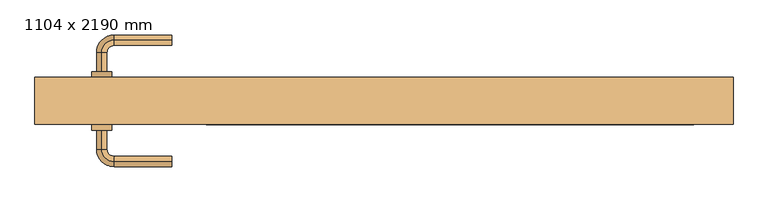
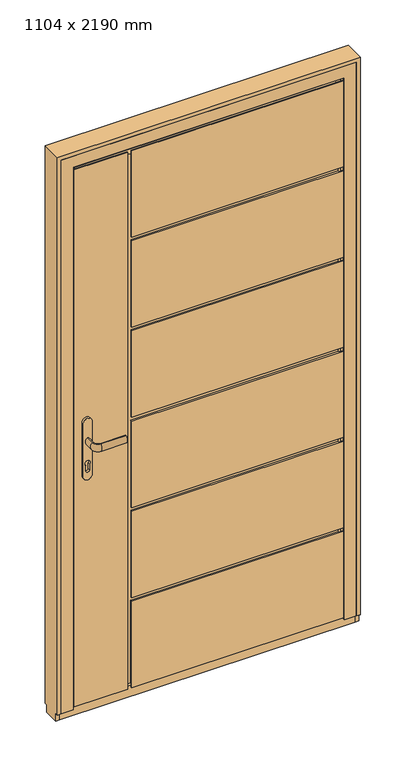
"""IFC4 building model written with IfcOpenShell, lengths in millimetres: door geometry, 1104 x 2190 mm."""

from ifc_helpers import new_model, si_unit, point, frame, frame_2d, origin, place, context, project, spatial, polyline, circle_curve, ellipse_curve, trimmed, segment, composite_curve, outline, extrude, faceted_brep, source, transform, mapped, element, save
from ifc_brep_helpers import plane_surface, revolved_surface, extruded_surface, advanced_brep


def door_1104_x_2190_mm_4e9de5db(model_context):
    return source(origin(), model_context, "Body", "SolidModel", [
        advanced_brep(
        [(-458.7, -104.0, 1064.0), (-458.7, -104.0, 1036.0), (-345.2, -155.0, 1064.0), (-345.2, -155.0, 1036.0), (-458.7, -135.0, 1064.0), (-458.7, -135.0, 1036.0), (-438.7, -155.0, 1036.0), (-438.7, -155.0, 1064.0)],
        [
            (0, 1, ellipse_curve(frame((-458.7, -104.0, 1050.0), z_axis=(0.0, 1.0, 0.0), x_axis=(0.0, 0.0, -1.0)), 14.0, 8.5)),
            (1, 0, ellipse_curve(frame((-458.7, -104.0, 1050.0), z_axis=(0.0, 1.0, 0.0), x_axis=(0.0, 0.0, -1.0)), 14.0, 8.5)),
            (2, 3, ellipse_curve(frame((-345.2, -155.0, 1050.0), z_axis=(1.0, 0.0, 0.0), x_axis=(0.0, 0.0, -1.0)), 14.0, 8.5)),
            (3, 2, ellipse_curve(frame((-345.2, -155.0, 1050.0), z_axis=(1.0, 0.0, 0.0), x_axis=(0.0, 0.0, -1.0)), 14.0, 8.5)),
            (0, 4),
            (4, 5, ellipse_curve(frame((-458.7, -135.0, 1050.0), z_axis=(0.0, 1.0, 0.0), x_axis=(0.0, 0.0, -1.0)), 14.0, 8.5)),
            (5, 1),
            (5, 4, ellipse_curve(frame((-458.7, -135.0, 1050.0), z_axis=(0.0, 1.0, 0.0), x_axis=(0.0, 0.0, -1.0)), 14.0, 8.5)),
            (6, 7, ellipse_curve(frame((-438.7, -155.0, 1050.0), z_axis=(1.0, 0.0, 0.0), x_axis=(0.0, 0.0, -1.0)), 14.0, 8.5)),
            (7, 2),
            (3, 6),
            (7, 6, ellipse_curve(frame((-438.7, -155.0, 1050.0), z_axis=(1.0, 0.0, 0.0), x_axis=(0.0, 0.0, -1.0)), 14.0, 8.5)),
            (6, 5, circle_curve(frame((-438.7, -135.0, 1036.0), z_axis=(0.0, 0.0, -1.0), x_axis=(-1.0, 0.0, 0.0)), 20.0)),
            (4, 7, circle_curve(frame((-438.7, -135.0, 1064.0), z_axis=(0.0, 0.0, 1.0), x_axis=(-1.0, 0.0, 0.0)), 20.0)),
        ],
        [
            plane_surface(frame((-458.7, -104.0, 1050.0), z_axis=(0.0, 1.0, 0.0), x_axis=(0.0, 0.0, 1.0))),
            plane_surface(frame((-345.2, -155.0, 1050.0), z_axis=(1.0, 0.0, 0.0), x_axis=(0.0, 0.0, 1.0))),
            extruded_surface(trimmed(ellipse_curve(frame((-458.7, -135.0, 1050.0), z_axis=(0.0, 1.0, 0.0), x_axis=(0.0, 0.0, -1.0)), 14.0, 8.5), [point((-458.7, -135.0, 1064.0))], [point((-458.7, -135.0, 1036.0))], True, "CARTESIAN"), (0.0, 31.0, 0.0), 31.0),
            extruded_surface(trimmed(ellipse_curve(frame((-458.7, -135.0, 1050.0), z_axis=(0.0, 1.0, 0.0), x_axis=(0.0, 0.0, -1.0)), 14.0, 8.5), [point((-458.7, -135.0, 1036.0))], [point((-458.7, -135.0, 1064.0))], True, "CARTESIAN"), (0.0, 31.0, 0.0), 31.0),
            extruded_surface(trimmed(ellipse_curve(frame((-345.2, -155.0, 1050.0), z_axis=(-1.0, 0.0, 0.0), x_axis=(0.0, 0.0, -1.0)), 14.0, 8.5), [point((-345.2, -155.0, 1064.0))], [point((-345.2, -155.0, 1036.0))], True, "CARTESIAN"), (-93.5, 0.0, 0.0), 93.5),
            extruded_surface(trimmed(ellipse_curve(frame((-345.2, -155.0, 1050.0), z_axis=(-1.0, 0.0, 0.0), x_axis=(0.0, 0.0, -1.0)), 14.0, 8.5), [point((-345.2, -155.0, 1036.0))], [point((-345.2, -155.0, 1064.0))], True, "CARTESIAN"), (-93.5, 0.0, 0.0), 93.5),
            revolved_surface(trimmed(ellipse_curve(frame((-458.7, -135.0, 1050.0), z_axis=(0.0, 1.0, 0.0), x_axis=(0.0, 0.0, -1.0)), 14.0, 8.5), [point((-458.7, -135.0, 1064.0))], [point((-458.7, -135.0, 1036.0))], True, "CARTESIAN"), (-438.7, -135.0, 1050.0), (0.0, 0.0, 1.0)),
            revolved_surface(trimmed(ellipse_curve(frame((-458.7, -135.0, 1050.0), z_axis=(0.0, 1.0, 0.0), x_axis=(0.0, 0.0, -1.0)), 14.0, 8.5), [point((-458.7, -135.0, 1036.0))], [point((-458.7, -135.0, 1064.0))], True, "CARTESIAN"), (-438.7, -135.0, 1050.0), (0.0, 0.0, 1.0)),
        ],
        [
            (0, [[1, 2]]),
            (1, [[3, 4]]),
            (2, [[-1, 5, 6, 7]]),
            (3, [[-2, -7, 8, -5]]),
            (4, [[9, 10, -4, 11]]),
            (5, [[12, -11, -3, -10]]),
            (6, [[13, -6, 14, -9]]),
            (7, [[-14, -8, -13, -12]]),
        ],
    ),
        extrude(outline(composite_curve([segment(polyline([(1124.5, -475.2), (914.5, -475.2)]), True, "CONTINUOUS"), segment(trimmed(circle_curve(frame_2d((914.5, -458.7)), 16.5), [point((914.5, -475.2))], [point((914.5, -442.2))], False, "CARTESIAN"), True, "CONTINUOUS"), segment(polyline([(914.5, -442.2), (1124.5, -442.2)]), True, "CONTINUOUS"), segment(trimmed(circle_curve(frame_2d((1124.5, -458.7)), 16.5), [point((1124.5, -442.2))], [point((1124.5, -475.2))], False, "CARTESIAN"), True, "CONTINUOUS")], self_intersect=False), holes=[composite_curve([segment(trimmed(circle_curve(frame_2d((963.5537881, -458.7)), 10.0), [point((956.4123597, -465.7))], [point((956.4123597, -451.7))], True, "CARTESIAN"), True, "CONTINUOUS"), segment(polyline([(956.4123597, -451.7), (935.5537881, -451.7)]), True, "CONTINUOUS"), segment(trimmed(circle_curve(frame_2d((935.5537881, -458.7)), 7.0), [point((935.5537881, -451.7))], [point((935.5537881, -465.7))], True, "CARTESIAN"), True, "CONTINUOUS"), segment(polyline([(935.5537881, -465.7), (956.4123597, -465.7)]), True, "CONTINUOUS")], self_intersect=False)]), frame((0.0, -104.0, 0.0), z_axis=(0.0, 1.0, 0.0), x_axis=(0.0, 0.0, 1.0)), (0.0, 0.0, 1.0), 9.0),
        advanced_brep(
        [(-458.7, -9.0, 1064.0), (-458.7, -9.0, 1036.0), (-345.2, 42.0, 1064.0), (-345.2, 42.0, 1036.0), (-458.7, 22.0, 1036.0), (-458.7, 22.0, 1064.0), (-438.7, 42.0, 1036.0), (-438.7, 42.0, 1064.0)],
        [
            (0, 1, ellipse_curve(frame((-458.7, -9.0, 1050.0), z_axis=(0.0, -1.0, 0.0), x_axis=(0.0, 0.0, -1.0)), 14.0, 8.5)),
            (1, 0, ellipse_curve(frame((-458.7, -9.0, 1050.0), z_axis=(0.0, -1.0, 0.0), x_axis=(0.0, 0.0, -1.0)), 14.0, 8.5)),
            (2, 3, ellipse_curve(frame((-345.2, 42.0, 1050.0), z_axis=(1.0, 0.0, 0.0), x_axis=(0.0, 0.0, -1.0)), 14.0, 8.5)),
            (3, 2, ellipse_curve(frame((-345.2, 42.0, 1050.0), z_axis=(1.0, 0.0, 0.0), x_axis=(0.0, 0.0, -1.0)), 14.0, 8.5)),
            (1, 4),
            (4, 5, ellipse_curve(frame((-458.7, 22.0, 1050.0), z_axis=(0.0, -1.0, 0.0), x_axis=(0.0, 0.0, -1.0)), 14.0, 8.5)),
            (5, 0),
            (5, 4, ellipse_curve(frame((-458.7, 22.0, 1050.0), z_axis=(0.0, -1.0, 0.0), x_axis=(0.0, 0.0, -1.0)), 14.0, 8.5)),
            (6, 3),
            (2, 7),
            (7, 6, ellipse_curve(frame((-438.7, 42.0, 1050.0), z_axis=(1.0, 0.0, 0.0), x_axis=(0.0, 0.0, -1.0)), 14.0, 8.5)),
            (6, 7, ellipse_curve(frame((-438.7, 42.0, 1050.0), z_axis=(1.0, 0.0, 0.0), x_axis=(0.0, 0.0, -1.0)), 14.0, 8.5)),
            (7, 5, circle_curve(frame((-438.7, 22.0, 1064.0), z_axis=(0.0, 0.0, 1.0), x_axis=(-1.0, 0.0, 0.0)), 20.0)),
            (4, 6, circle_curve(frame((-438.7, 22.0, 1036.0), z_axis=(0.0, 0.0, -1.0), x_axis=(-1.0, 0.0, 0.0)), 20.0)),
        ],
        [
            plane_surface(frame((-458.7, -9.0, 1050.0), z_axis=(0.0, -1.0, 0.0), x_axis=(0.0, 0.0, 1.0))),
            plane_surface(frame((-345.2, 42.0, 1050.0), z_axis=(1.0, 0.0, 0.0), x_axis=(0.0, 0.0, 1.0))),
            extruded_surface(trimmed(ellipse_curve(frame((-458.7, -9.0, 1050.0), z_axis=(0.0, 1.0, 0.0), x_axis=(0.0, 0.0, -1.0)), 14.0, 8.5), [point((-458.7, -9.0, 1064.0))], [point((-458.7, -9.0, 1036.0))], True, "CARTESIAN"), (0.0, 31.0, 0.0), 31.0),
            extruded_surface(trimmed(ellipse_curve(frame((-458.7, -9.0, 1050.0), z_axis=(0.0, 1.0, 0.0), x_axis=(0.0, 0.0, -1.0)), 14.0, 8.5), [point((-458.7, -9.0, 1036.0))], [point((-458.7, -9.0, 1064.0))], True, "CARTESIAN"), (0.0, 31.0, 0.0), 31.0),
            extruded_surface(trimmed(ellipse_curve(frame((-438.7, 42.0, 1050.0), z_axis=(1.0, 0.0, 0.0), x_axis=(0.0, 0.0, -1.0)), 14.0, 8.5), [point((-438.7, 42.0, 1064.0))], [point((-438.7, 42.0, 1036.0))], True, "CARTESIAN"), (93.5, 0.0, 0.0), 93.5),
            extruded_surface(trimmed(ellipse_curve(frame((-438.7, 42.0, 1050.0), z_axis=(1.0, 0.0, 0.0), x_axis=(0.0, 0.0, -1.0)), 14.0, 8.5), [point((-438.7, 42.0, 1036.0))], [point((-438.7, 42.0, 1064.0))], True, "CARTESIAN"), (93.5, 0.0, 0.0), 93.5),
            revolved_surface(trimmed(ellipse_curve(frame((-458.7, 22.0, 1050.0), z_axis=(0.0, 1.0, 0.0), x_axis=(0.0, 0.0, -1.0)), 14.0, 8.5), [point((-458.7, 22.0, 1064.0))], [point((-458.7, 22.0, 1036.0))], True, "CARTESIAN"), (-438.7, 22.0, 1050.0), (0.0, 0.0, 1.0)),
            revolved_surface(trimmed(ellipse_curve(frame((-458.7, 22.0, 1050.0), z_axis=(0.0, 1.0, 0.0), x_axis=(0.0, 0.0, -1.0)), 14.0, 8.5), [point((-458.7, 22.0, 1036.0))], [point((-458.7, 22.0, 1064.0))], True, "CARTESIAN"), (-438.7, 22.0, 1050.0), (0.0, 0.0, 1.0)),
        ],
        [
            (0, [[1, 2]]),
            (1, [[3, 4]]),
            (2, [[5, 6, 7, -2]]),
            (3, [[-7, 8, -5, -1]]),
            (4, [[9, -3, 10, 11]]),
            (5, [[-10, -4, -9, 12]]),
            (6, [[-11, 13, -6, 14]]),
            (7, [[-12, -14, -8, -13]]),
        ],
    ),
        extrude(outline(composite_curve([segment(polyline([(1124.5, -475.2), (914.5, -475.2)]), True, "CONTINUOUS"), segment(trimmed(circle_curve(frame_2d((914.5, -458.7)), 16.5), [point((914.5, -475.2))], [point((914.5, -442.2))], False, "CARTESIAN"), True, "CONTINUOUS"), segment(polyline([(914.5, -442.2), (1124.5, -442.2)]), True, "CONTINUOUS"), segment(trimmed(circle_curve(frame_2d((1124.5, -458.7)), 16.5), [point((1124.5, -442.2))], [point((1124.5, -475.2))], False, "CARTESIAN"), True, "CONTINUOUS")], self_intersect=False), holes=[composite_curve([segment(trimmed(circle_curve(frame_2d((963.5537881, -458.7)), 10.0), [point((956.4123597, -465.7))], [point((956.4123597, -451.7))], True, "CARTESIAN"), True, "CONTINUOUS"), segment(polyline([(956.4123597, -451.7), (935.5537881, -451.7)]), True, "CONTINUOUS"), segment(trimmed(circle_curve(frame_2d((935.5537881, -458.7)), 7.0), [point((935.5537881, -451.7))], [point((935.5537881, -465.7))], True, "CARTESIAN"), True, "CONTINUOUS"), segment(polyline([(935.5537881, -465.7), (956.4123597, -465.7)]), True, "CONTINUOUS")], self_intersect=False)]), frame((0.0, -18.0, 0.0), z_axis=(0.0, 1.0, 0.0), x_axis=(0.0, 0.0, 1.0)), (0.0, 0.0, 1.0), 9.0),
        faceted_brep([(-288.7, -25.0, 366.5833337), (478.7, -25.0, 366.5833337), (478.7, -25.0, 351.5833337), (-288.7, -25.0, 351.5833337), (-288.7, -25.0, 35.0), (-303.7, -25.0, 35.0), (-303.7, -25.0, 2109.5000003), (-288.7, -25.0, 2109.5000003), (-288.7, -25.0, 1792.916667), (478.7, -25.0, 1792.916667), (478.7, -25.0, 1777.916667), (-288.7, -25.0, 1777.916667), (-288.7, -25.0, 1436.3333337), (478.7, -25.0, 1436.3333337), (478.7, -25.0, 1421.3333337), (-288.7, -25.0, 1421.3333337), (-288.7, -25.0, 1079.7500004), (478.7, -25.0, 1079.7500004), (478.7, -25.0, 1064.7500004), (-288.7, -25.0, 1064.7500004), (-288.7, -25.0, 723.166667), (478.7, -25.0, 723.166667), (478.7, -25.0, 708.166667), (-288.7, -25.0, 708.166667), (-288.7, -18.0, 708.166667), (-288.7, -18.0, 366.5833337), (478.7, -18.0, 708.166667), (478.7, -27.0002302, 2109.5000003), (478.7, -27.0002302, 35.0), (478.7, -19.9979528, 35.0), (478.7, -19.9979528, 24.0), (478.7, -18.0, 24.0), (478.7, -18.0, 351.5833337), (478.7, -18.0, 366.5833337), (478.7, -18.0, 723.166667), (478.7, -18.0, 1064.7500004), (478.7, -18.0, 1079.7500004), (478.7, -18.0, 1421.3333337), (478.7, -18.0, 1436.3333337), (478.7, -18.0, 1777.916667), (478.7, -18.0, 1792.916667), (478.7, -18.0, 2109.5000003), (-288.7, -18.0, 723.166667), (-288.7, -18.0, 1064.7500004), (-288.7, -18.0, 1079.7500004), (-288.7, -18.0, 1421.3333337), (-303.7, -19.9979528, 35.0), (-303.7, -19.9979528, 24.0), (-303.7, -18.0, 24.0), (-303.7, -18.0, 2109.5000003), (-478.7, -27.0002302, 35.0), (-478.7, -19.9979528, 35.0), (-288.7, -19.9979528, 35.0), (-288.7, -18.0, 351.5833337), (-288.7, -18.0, 24.0), (-288.7, -19.9979528, 24.0), (-478.7, -19.9979528, 24.0), (-478.7, -18.0, 24.0), (-478.7, -18.0, 2109.5000003), (-288.7, -18.0, 1436.3333337), (-288.7, -18.0, 1777.916667), (-288.7, -18.0, 1792.916667), (-288.7, -18.0, 2109.5000003), (503.7, -95.0, 10.0000003), (-288.7, -95.0, 10.0000003), (-288.7, -92.0, 10.0000003), (503.7, -92.0, 10.0000003), (-503.7, -92.0, 10.0000003), (-303.7, -92.0, 10.0000003), (-303.7, -95.0, 10.0000003), (-503.7, -95.0, 10.0000003), (503.7, -95.0, 366.5833337), (503.7, -92.0, 366.5833337), (503.7, -92.0, 708.166667), (503.7, -95.0, 708.166667), (503.7, -95.0, 1079.7500004), (503.7, -92.0, 1079.7500004), (503.7, -92.0, 1421.3333337), (503.7, -95.0, 1421.3333337), (503.7, -95.0, 723.166667), (503.7, -92.0, 723.166667), (503.7, -92.0, 1064.7500004), (503.7, -95.0, 1064.7500004), (503.7, -95.0, 1436.3333337), (503.7, -92.0, 1436.3333337), (503.7, -92.0, 1777.916667), (503.7, -95.0, 1777.916667), (503.7, -95.0, 2134.5000003), (503.7, -95.0, 1792.916667), (503.7, -92.0, 1792.916667), (503.7, -92.0, 2134.5000003), (503.7, -92.0, 351.5833337), (503.7, -95.0, 351.5833337), (-288.7, -92.0, 25.5), (488.2, -92.0, 25.5), (488.2, -92.0, 351.5833337), (488.2, -92.0, 366.5833337), (488.2, -92.0, 708.166667), (488.2, -92.0, 1079.7500004), (488.2, -92.0, 1421.3333337), (488.2, -92.0, 723.166667), (488.2, -92.0, 1064.7500004), (-488.2, -92.0, 25.5), (-303.7, -92.0, 25.5), (-503.7, -92.0, 2134.5000003), (-303.7, -92.0, 2134.5000003), (-303.7, -92.0, 2119.0000003), (-488.2, -92.0, 2119.0000003), (488.2, -92.0, 1436.3333337), (488.2, -92.0, 1777.916667), (488.2, -92.0, 1792.916667), (488.2, -92.0, 2119.0000003), (-288.7, -92.0, 2119.0000003), (-288.7, -92.0, 2134.5000003), (-288.7, -88.0, 351.5833337), (-288.7, -88.0, 25.5), (-288.7, -95.0, 351.5833337), (-303.7, -95.0, 2134.5000003), (-503.7, -95.0, 2134.5000003), (-288.7, -95.0, 708.166667), (-288.7, -95.0, 366.5833337), (-288.7, -95.0, 1421.3333337), (-288.7, -95.0, 1079.7500004), (-288.7, -95.0, 1064.7500004), (-288.7, -95.0, 723.166667), (-288.7, -95.0, 1777.916667), (-288.7, -95.0, 1436.3333337), (-288.7, -95.0, 2134.5000003), (-288.7, -95.0, 1792.916667), (-303.7, -88.0, 2119.0000003), (-303.7, -88.0, 25.5), (-478.7, -27.0002302, 2109.5000003), (488.2, -27.0002302, 2119.0000003), (488.2, -27.0002302, 25.5), (-488.2, -27.0002302, 25.5), (-488.2, -27.0002302, 2119.0000003), (488.2, -88.0, 1792.916667), (488.2, -88.0, 1777.916667), (488.2, -88.0, 1436.3333337), (488.2, -88.0, 1421.3333337), (488.2, -88.0, 1079.7500004), (488.2, -88.0, 1064.7500004), (488.2, -88.0, 723.166667), (488.2, -88.0, 708.166667), (488.2, -88.0, 366.5833337), (488.2, -88.0, 351.5833337), (-288.7, -88.0, 1777.916667), (-288.7, -88.0, 1792.916667), (-288.7, -88.0, 2119.0000003), (-288.7, -88.0, 366.5833337), (-288.7, -88.0, 708.166667), (-288.7, -88.0, 723.166667), (-288.7, -88.0, 1064.7500004), (-288.7, -88.0, 1079.7500004), (-288.7, -88.0, 1421.3333337), (-288.7, -88.0, 1436.3333337)], [[[0, 1, 2, 3, 4, 5, 6, 7, 8, 9, 10, 11, 12, 13, 14, 15, 16, 17, 18, 19, 20, 21, 22, 23]], [[23, 24, 25, 0]], [[23, 22, 26, 24]], [[27, 28, 29, 30, 31, 32, 2, 1, 33, 26, 22, 21, 34, 35, 18, 17, 36, 37, 14, 13, 38, 39, 10, 9, 40, 41]], [[42, 34, 21, 20]], [[19, 43, 42, 20]], [[19, 18, 35, 43]], [[44, 36, 17, 16]], [[15, 45, 44, 16]], [[5, 46, 47, 48, 49, 6]], [[28, 50, 51, 46, 5, 4, 52, 29]], [[53, 54, 55, 52, 4, 3]], [[3, 2, 32, 53]], [[25, 33, 1, 0]], [[29, 52, 55, 30]], [[56, 47, 46, 51]], [[30, 55, 54, 31]], [[57, 48, 47, 56]], [[36, 44, 45, 37]], [[34, 42, 43, 35]], [[33, 25, 24, 26]], [[54, 53, 32, 31]], [[58, 49, 48, 57]], [[38, 59, 60, 39]], [[41, 40, 61, 62]], [[63, 64, 65, 66]], [[67, 68, 69, 70]], [[71, 72, 73, 74]], [[75, 76, 77, 78]], [[79, 80, 81, 82]], [[83, 84, 85, 86]], [[87, 88, 89, 90]], [[66, 91, 92, 63]], [[65, 93, 94, 95, 91, 66]], [[72, 96, 97, 73]], [[76, 98, 99, 77]], [[80, 100, 101, 81]], [[102, 103, 68, 67, 104, 105, 106, 107]], [[84, 108, 109, 85]], [[90, 89, 110, 111, 112, 113]], [[114, 115, 93, 65, 64, 116]], [[70, 69, 117, 118]], [[63, 92, 116, 64]], [[74, 119, 120, 71]], [[78, 121, 122, 75]], [[82, 123, 124, 79]], [[86, 125, 126, 83]], [[87, 127, 128, 88]], [[70, 118, 104, 67]], [[129, 106, 105, 117, 69, 68, 103, 130]], [[58, 57, 56, 51, 50, 131]], [[132, 133, 134, 135], [131, 50, 28, 27]], [[111, 110, 136, 137, 109, 108, 138, 139, 99, 98, 140, 141, 101, 100, 142, 143, 97, 96, 144, 145, 95, 94, 133, 132]], [[94, 93, 115, 130, 103, 102, 134, 133]], [[135, 134, 102, 107]], [[146, 137, 136, 147, 148, 129, 130, 115, 114, 145, 144, 149, 150, 143, 142, 151, 152, 141, 140, 153, 154, 139, 138, 155]], [[153, 122, 121, 154]], [[153, 140, 98, 76, 75, 122]], [[123, 82, 81, 101, 141, 152]], [[151, 124, 123, 152]], [[151, 142, 100, 80, 79, 124]], [[119, 74, 73, 97, 143, 150]], [[149, 120, 119, 150]], [[149, 144, 96, 72, 71, 120]], [[116, 92, 91, 95, 145, 114]], [[15, 14, 37, 45]], [[59, 38, 13, 12]], [[11, 60, 59, 12]], [[11, 10, 39, 60]], [[61, 40, 9, 8]], [[8, 7, 62, 61]], [[125, 86, 85, 109, 137, 146]], [[128, 127, 113, 112, 148, 147]], [[121, 78, 77, 99, 139, 154]], [[155, 138, 108, 84, 83, 126]], [[155, 126, 125, 146]], [[147, 136, 110, 89, 88, 128]], [[90, 113, 127, 87]], [[118, 117, 105, 104]], [[132, 135, 107, 106, 129, 148, 112, 111]], [[27, 41, 62, 7, 6, 49, 58, 131]]]),
        faceted_brep([(-552.25, -95.0, 0.0), (-552.25, -85.9997571, 0.0), (-507.75, -85.9997571, 0.0), (-507.75, -95.0, 0.0), (-498.25, -22.5000042, 0.0), (-498.25, -27.0, 0.0), (-552.25, -27.0, 0.0), (-552.25, -18.0, 0.0), (-482.75, -18.0, 0.0), (-482.75, -22.5000042, 0.0), (552.25, -18.0, 0.0), (552.25, -27.0, 0.0), (498.25, -27.0, 0.0), (498.25, -22.5000042, 0.0), (482.75, -22.5000042, 0.0), (482.75, -18.0, 0.0), (507.75, -85.9997571, 0.0), (552.25, -85.9997571, 0.0), (552.25, -95.0, 0.0), (507.75, -95.0, 0.0), (-552.25, -27.0, -30.0), (-552.25, -85.9997571, -30.0), (-552.25, -95.0, 2189.5), (-552.25, -18.0, 2189.5), (-507.75, -95.0, 2145.0), (507.75, -95.0, 2145.0), (552.25, -95.0, 2189.5), (552.25, -18.0, 2189.5), (552.25, -85.9997571, -30.0), (552.25, -27.0, -30.0), (482.75, -18.0, 2120.0), (-482.75, -18.0, 2120.0), (-498.25, -86.0, 2135.5), (-498.25, -86.0, 14.5), (-498.25, -27.0, 14.5), (-498.25, -22.5000042, 2135.5), (498.25, -22.5000042, 2135.5), (498.25, -86.0, 2135.5), (498.25, -27.0, 14.5), (498.25, -86.0, 14.5), (-507.75, -86.0, 2145.0), (507.75, -86.0, 2145.0), (-482.75, -22.5000042, 2120.0), (482.75, -22.5000042, 2120.0)], [[[0, 1, 2, 3]], [[4, 5, 6, 7, 8, 9]], [[10, 11, 12, 13, 14, 15]], [[16, 17, 18, 19]], [[7, 6, 20, 21, 1, 0, 22, 23]], [[3, 24, 25, 19, 18, 26, 22, 0]], [[22, 26, 27, 23]], [[18, 17, 28, 29, 11, 10, 27, 26]], [[7, 23, 27, 10, 15, 30, 31, 8]], [[32, 33, 34, 5, 4, 35]], [[35, 36, 37, 32]], [[36, 13, 12, 38, 39, 37]], [[40, 24, 3, 2]], [[16, 41, 40, 2, 1, 21, 28, 17], [37, 39, 33, 32]], [[9, 42, 43, 14, 13, 36, 35, 4]], [[8, 31, 42, 9]], [[24, 40, 41, 25]], [[30, 43, 42, 31]], [[19, 25, 41, 16]], [[14, 43, 30, 15]], [[20, 6, 5, 34, 38, 12, 11, 29]], [[39, 38, 34, 33]], [[20, 29, 28, 21]]]),
        faceted_brep([(-552.25, -86.0, -30.0), (-567.25, -86.0, -30.0), (-567.25, -27.0, -30.0), (-552.25, -27.0, -30.0), (-552.25, -95.0, 2189.5), (-552.25, -95.0, 0.0), (-552.25, -86.0, 0.0), (-552.25, -27.0, 0.0), (-552.25, -18.0, 0.0), (-552.25, -18.0, 2189.5), (-567.25, -27.0, 0.0), (567.25, -27.0, 0.0), (567.25, -27.0, -30.0), (552.25, -27.0, -30.0), (552.25, -27.0, 0.0), (-567.25, -18.0, 2204.5), (-567.25, -18.0, 0.0), (-567.25, -86.0, 0.0), (-567.25, -95.0, 0.0), (-567.25, -95.0, 2204.5), (552.25, -86.0, 0.0), (552.25, -86.0, -30.0), (567.25, -86.0, -30.0), (567.25, -86.0, 0.0), (552.25, -18.0, 2189.5), (552.25, -18.0, 0.0), (552.25, -95.0, 0.0), (552.25, -95.0, 2189.5), (567.25, -95.0, 0.0), (567.25, -95.0, 2204.5), (567.25, -18.0, 0.0), (567.25, -18.0, 2204.5)], [[[0, 1, 2, 3]], [[4, 5, 6, 0, 3, 7, 8, 9]], [[7, 3, 2, 10]], [[11, 12, 13, 14]], [[15, 16, 10, 2, 1, 17, 18, 19]], [[17, 1, 0, 6]], [[20, 21, 22, 23]], [[24, 25, 14, 13, 21, 20, 26, 27]], [[27, 26, 28, 29, 19, 18, 5, 4]], [[6, 5, 18, 17]], [[23, 28, 26, 20]], [[22, 21, 13, 12]], [[10, 16, 8, 7]], [[14, 25, 30, 11]], [[9, 8, 16, 15, 31, 30, 25, 24]], [[29, 28, 23, 22, 12, 11, 30, 31]], [[9, 24, 27, 4]], [[19, 29, 31, 15]]]),
    ])


if __name__ == "__main__":
    model = new_model("IFC4")
    model_context = context("Model", 3, world=origin())
    ifc_project = project(units=[si_unit("LENGTHUNIT", "METRE", prefix="MILLI")], contexts=[model_context])
    site = spatial("IfcSite", under=ifc_project)
    building = spatial("IfcBuilding", under=site)
    placement = place(None, origin())
    door_1104_x_2190_mm_shape = door_1104_x_2190_mm_4e9de5db(model_context)
    element("IfcDoor", 1, ObjectType="1104 x 2190 mm", at=placement, inside=building, context=model_context, shape_type="MappedRepresentation", body=[
        mapped(door_1104_x_2190_mm_shape, transform((0.0, 0.0, 0.0), x_axis=(1.0, 0.0, 0.0), y_axis=(0.0, 1.0, 0.0), z_axis=(0.0, 0.0, 1.0))),
    ])
    save(model, "model.ifc")

# Revit data of these elements
# Type "1104 x 2190 mm"
#   Type Mark = "28"
#   Water resistance = "up to Class E900, EN 12208:2001"
#   Uniclass2015Version = "v1.21"
#   Uniclass2015Reference = "Ss_25_30_20_30"
#   Uniclass2015Description = "Frame and door leaf system"
#   URL = "www.aluprof.eu"
#   Type IFC Predefined Type = "USERDEFINED"
#   Right-hand / Left-hand door [instance default] = ""
#   Resistance to wind load = "up to Class C5/B5, EN 12210:2001"
#   Insert type = "ST"
#   Hardware [instance default] = ""
#   Product page = "https://aluprof.eu/en/architects/offer/window-and-door-systems/panel-doors#visualisation"
#   Operation = "SinglePanelOutwardOpening"
#   Opening type = "Outward"
#   NBSReference = "25-50-20/125"
#   NBSDescription = "Frame and door leaf system"
#   Important = "The actual acceptable construction dimensions are dependent on the selection of profiles and hardware, glazing type, construction weight and the construction’s operating conditions. These should be determined by a suitably qualified person, and using ALUPROF’s calculation software"
#   IfcExportType = "USERDEFINED"
#   IfcExportAs = "IfcDoorType"
#   Handle type [instance default] = ""
#   Manufacturer = "ALUPROF"
#   Export Type to IFC As = "IfcDoorType"
#   Door sill type [instance default] = ""
#   Description = "External single-leaf panel door outward opening"
#   Model = "MB-86 ST Panel Door AD07"
#   Content of the recyclate in the material = "69.2"
#   COBie.Type.WarrantyDurationParts = ""
#   COBie.Type.Name = ""
#   COBie.Type.Manufacturer = "ALUPROF S.A."
#   COBie.Space.Name = ""
#   COBie.Floor.Name = ""
#   COBie.Facility.Name = ""
#   COBie.CreatedOn = ""
#   COBie.Component.WarrantyStartDate = ""
#   COBie.Component.Name = "MB-86 ST Panel Door AD07"
#   Burglar resistance = "RC2"
#   Air permeability = "up to Class 4, EN 12207:2001"
#   Width of the active leaf = 1007.4 mm
#   Placement in wall = 20 mm
#   Thickness = 77 mm
#   Height of the opening sash = 2124.5 mm
#   Handle Offset = 1050 mm
#   Glazing thickness = 48 mm
#   Rough Height = 2250.7 mm
#   Rough Width = 1134.5 mm
#   Height = 2189.5 mm
#   Width = 1104.5 mm
#   Construction depth = 77 mm
#   Clear opening width = 900 mm
#   Clear opening height = 2100 mm
#   Height of the array = 341.583 mm
#   Schedule No. [instance default] = 1
#   Handrail = no
#   IsExternal = yes
#   Handle = yes
#   Door closer [instance default] = no
#   Function = 1
#   COBie.Type = yes
#   COBie = yes
#   Access control [instance default] = no
#   Panel = element 260956
#   Wall Closure = (empty or 0)
